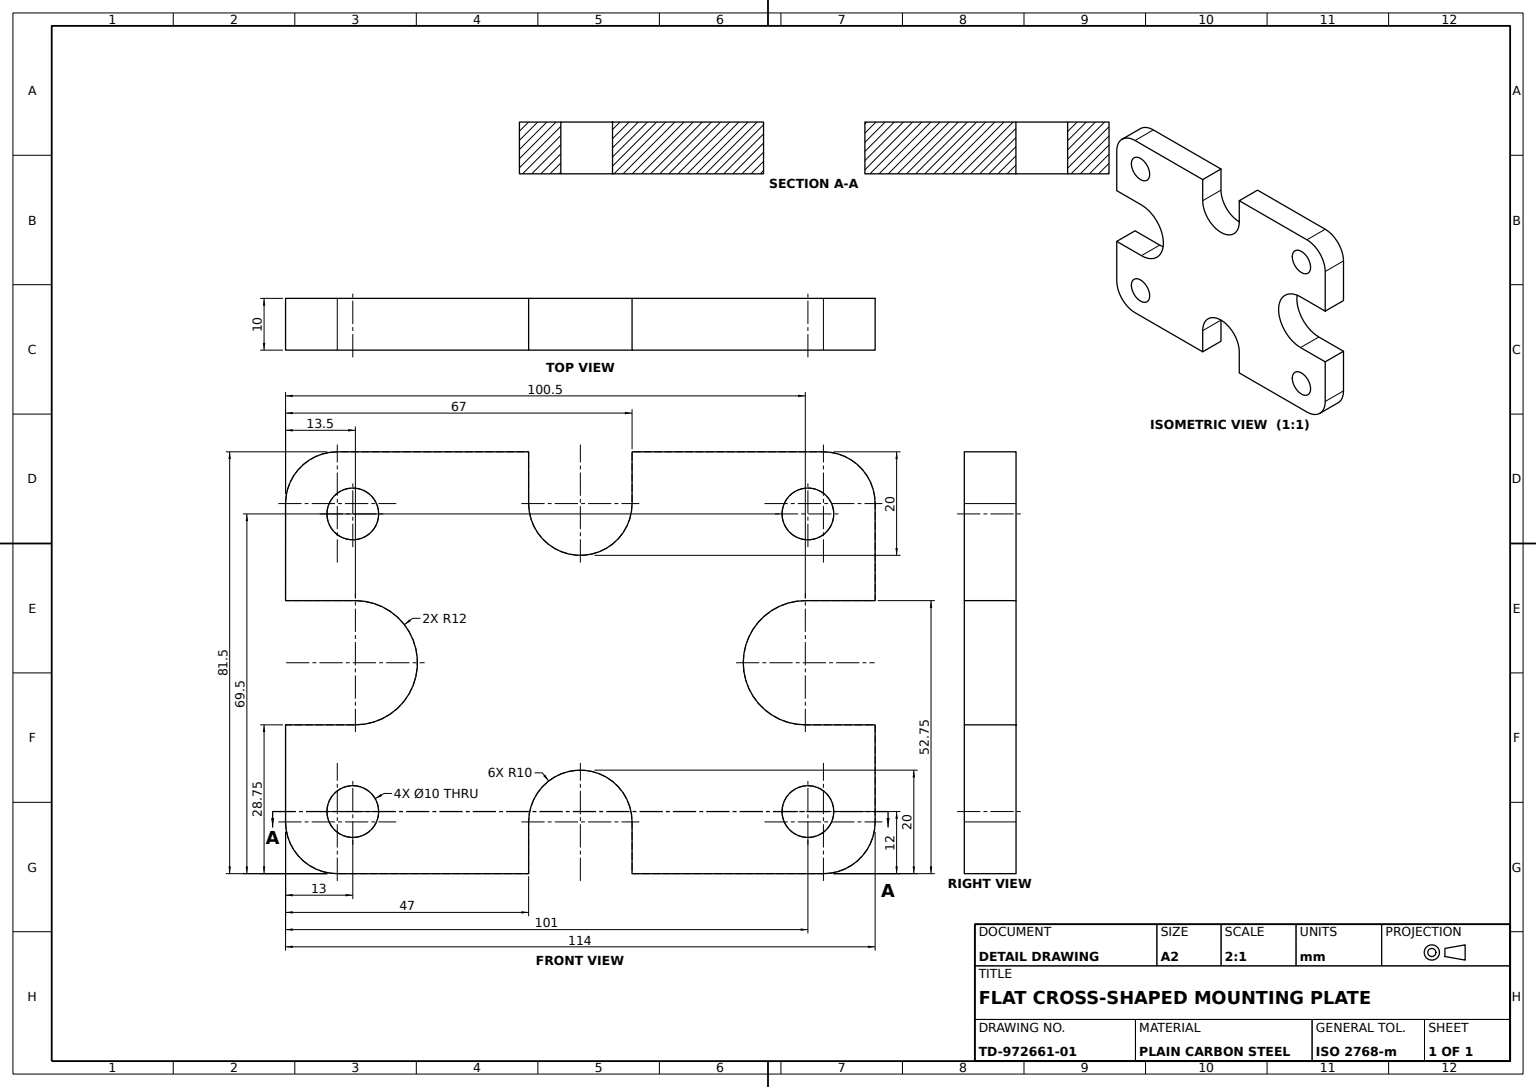
SolidWorks part; units mm, degrees
material "Plain Carbon Steel"
ref_plane "Front Plane" through (0, 0, 0) normal (0, 0, 1) x (1, 0, 0)
ref_plane "Top Plane" through (0, 0, 0) normal (0, 1, 0) x (1, 0, 0)
ref_plane "Right Plane" through (0, 0, 0) normal (1, 0, 0) x (0, 0, -1)
sketch "Bracket Profile Sketch" plane through (0, 0, 0) normal (0, 0, 1) x (1, 0, 0)
  line L0 (10, 0) -> (47, 0)
  line L1 (114, 10) -> (114, 28.75)
  line L2 (104, 81.5) -> (67, 81.5)
  line L3 (0, 71.5) -> (0, 52.75)
  line L4 (10, 0) -> (47, 0) construction
  line L5 (47, 0) -> (47, 10)
  line L6 (114, 10) -> (114, 28.75) construction
  line L7 (67, 10) -> (67, 0)
  line L8 (67, 0) -> (104, 0)
  line L9 (67, 81.5) -> (67, 71.5)
  line L11 (100.5, 52.75) -> (114, 52.75)
  line L12 (100.5, 28.75) -> (114, 28.75)
  line L13 (114, 52.75) -> (114, 71.5)
  line L14 (47, 71.5) -> (47, 81.5)
  line L15 (47, 81.5) -> (10, 81.5)
  line L16 (0, 52.75) -> (13.5, 52.75)
  line L17 (0, 71.5) -> (0, 81.5)
  line L18 (13.5, 28.75) -> (0, 28.75)
  line L19 (0, 28.75) -> (0, 10)
  line L20 (0, 81.5) -> (10, 81.5)
  line L21 (104, 81.5) -> (114, 81.5)
  line L22 (114, 81.5) -> (114, 71.5)
  line L23 (114, 10) -> (114, 0)
  line L24 (114, 0) -> (104, 0)
  line L25 (0, 10) -> (0, 0)
  line L26 (0, 0) -> (10, 0)
  arc A4 (67, 10) -> (47, 10) centre (57, 10) ccw
  arc A5 (100.5, 52.75) -> (100.5, 28.75) centre (100.5, 40.75) ccw
  arc A6 (47, 71.5) -> (67, 71.5) centre (57, 71.5) ccw
  arc A7 (13.5, 28.75) -> (13.5, 52.75) centre (13.5, 40.75) ccw
  point P13 (0, 0)
  dimension "D2" = 24
  dimension "D3" = 10
  dimension "D8" = 28.75
  dimension "D9" = 10
  dimension "D10" = 81.5
  dimension "D13" = 12
  dimension "D4" = 37
  dimension "D5" = 37
  dimension "D6" = 20
  dimension "D7" = 13.5
  dimension "D11" = 71.5
  dimension "D12" = 10
  dimension "D14" = 40.75
  dimension "D15" = 13.5
  dimension "D16" = 28.75
  dimension "D17" = 10
  dimension "D18" = 10
  dimension "D19" = 10
  dimension "D20" = 114
extrude "Bracket Plate" add sketch "Bracket Profile Sketch" along normal blind 10
sketch "Mounting Holes Sketch" plane through (0, 0, 10) normal (0, 0, 1) x (1, 0, 0)
  line L1 (0, 81.5) -> (0, 52.75) construction
  line L2 (114, 81.5) -> (67, 81.5) construction
  line L3 (114, 52.75) -> (114, 81.5) construction
  line L4 (0, 28.75) -> (0, 0) construction
  line L5 (0, 0) -> (47, 0) construction
  line L6 (114, 0) -> (114, 28.75) construction
  line L7 (67, 0) -> (114, 0) construction
  circle A0 centre (13, 69.5) radius 5
  circle A1 centre (101, 69.5) radius 5
  circle A2 centre (101, 12) radius 5
  circle A3 centre (13, 12) radius 5
  dimension "D1" = 10
  dimension "D2" = 10
  dimension "D3" = 10
  dimension "D4" = 10
  dimension "D5" = 12
  dimension "D6" = 13
  dimension "D7" = 12
  dimension "D8" = 13
  dimension "D9" = 13
  dimension "D10" = 12
  dimension "D11" = 13
  dimension "D12" = 12
extrude "Mounting Holes 4xØ10" cut sketch "Mounting Holes Sketch" against normal through all
fillet "Corner Fillets R10" radius 10 4 edges at (114, 0, 5) (114, 81.5, 5) (0, 0, 5) (0, 81.5, 5)
